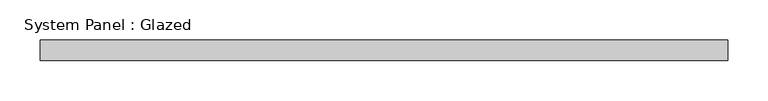
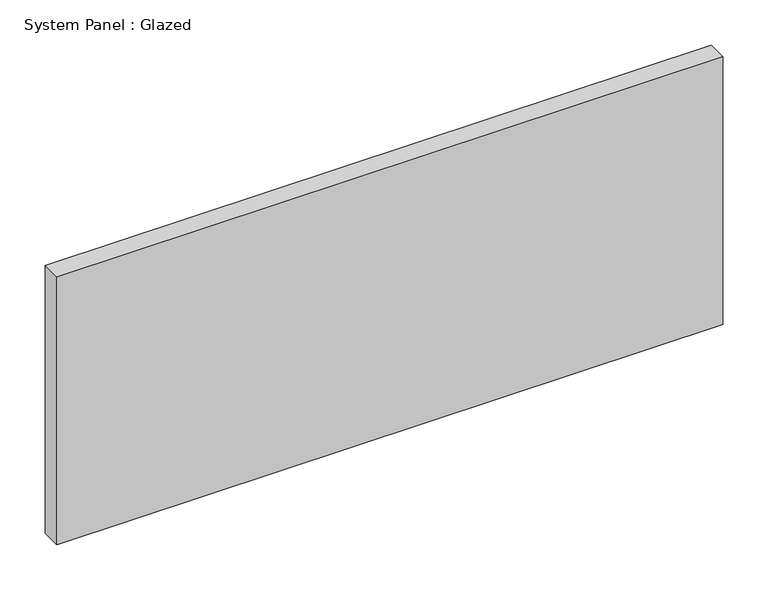
"""IFC4 building model written with IfcOpenShell, lengths in millimetres: plate geometry, System Panel : Glazed."""

from ifc_helpers import new_model, si_unit, origin, origin_with_axes, place, context, project, spatial, polyline, outline, extrude, source, transform, mapped, element, save


def system_panel_glazed_0c1cb5df(model_context):
    return source(origin(), model_context, "Body", "SweptSolid", [
        extrude(outline(polyline([(425.45, 19.05), (-425.45, 19.05), (-425.45, 44.45), (425.45, 44.45), (425.45, 19.05)])), origin_with_axes(), (0.0, 0.0, 1.0), 361.95),
    ])


if __name__ == "__main__":
    model = new_model("IFC4")
    model_context = context("Model", 3, world=origin())
    ifc_project = project(units=[si_unit("LENGTHUNIT", "METRE", prefix="MILLI")], contexts=[model_context])
    site = spatial("IfcSite", under=ifc_project)
    building = spatial("IfcBuilding", under=site)
    placement = place(None, origin())
    system_panel_glazed_shape = system_panel_glazed_0c1cb5df(model_context)
    element("IfcPlate", 1, ObjectType="System Panel : Glazed", at=placement, inside=building, context=model_context, shape_type="MappedRepresentation", body=[
        mapped(system_panel_glazed_shape, transform((0.0, 0.0, 0.0), x_axis=(1.0, 0.0, 0.0), y_axis=(0.0, 1.0, 0.0), z_axis=(0.0, 0.0, 1.0))),
    ])
    save(model, "model.ifc")

# Revit data of these elements
# Type "System Panel : Glazed"
#   Construction Type Id = "GSP4R"
#   Analytic Construction = "1/8 in Pilkington single glazing"
#   Visual Light Transmittance = 0.9
#   Solar Heat Gain Coefficient = 0.86
#   Heat Transfer Coefficient (U) = 1.18115 BTU/(h·ft²·°F)
#   Define Thermal Properties by = 1
# Element 1 (IfcPlate, "System Panel : Glazed")
#   Materials on its faces: "Glass"
# Materials
#   "Glass": class "Glass", colour RGB 0 128 192, transparency 0.75, Description = "Soda Lime Glass", Cost = 0
